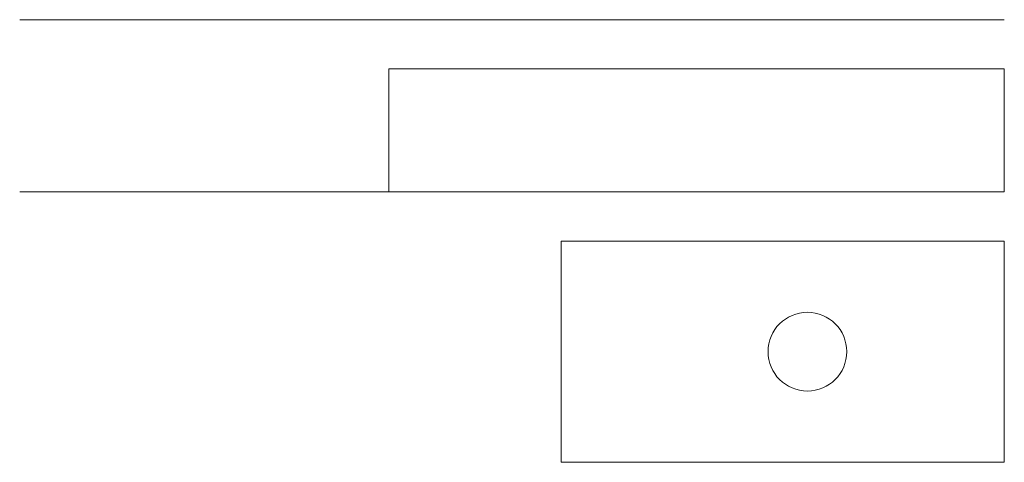
# Model space of a CAD drawing. Units: millimetres. Extents: x 50 to 250, y -55 to 35.
import ezdxf

# ---------------------------------------------------------------- set-up
doc = ezdxf.new("R2010")
doc.units = ezdxf.units.MM
doc.layers.add('M-CONS', color=8, linetype='Continuous', lineweight=18)

msp = doc.modelspace()

# ---------------------------------------------------------------- linework, layer by layer
at = {"layer": 'M-CONS', "extrusion": (0, -1, 0), "elevation": -35}
msp.add_lwpolyline([(70.37, -28.84), (250.37, -28.84), (250.37, -8.84), (187.37, 43.16), (70.37, 11.16)], dxfattribs=at)
at = {"layer": 'M-CONS', "extrusion": (0, -1, 0)}
msp.add_lwpolyline([(70.37, -28.84), (250.37, -28.84), (250.37, -8.84), (187.37, 43.16), (70.37, 11.16)], dxfattribs=at)
at = {"layer": 'M-CONS', "elevation": -28.84}
msp.add_lwpolyline([(160.37, -55), (250.37, -55), (250.37, -10), (160.37, -10)], close=True, dxfattribs=at)
at = {"layer": 'M-CONS'}
msp.add_polyline3d([(250.37, 0, -28.84), (250.37, 25, -28.84), (125.37, 25, -28.84), (125.37, 0, -28.84)], close=True, dxfattribs=at)
at = {"layer": 'M-CONS', "extrusion": (0, -1, 0)}
for centre, radius in [((70.37, -8.84, -35), 20), ((70.37, -8.84, -35), 8), ((70.37, -8.84), 20), ((70.37, -8.84), 8)]:
    msp.add_circle(centre, radius, dxfattribs=at)
at = {"layer": 'M-CONS'}
msp.add_circle((210.37, -32.5, -28.84), 8, dxfattribs=at)

doc.saveas('drawing.dxf')
